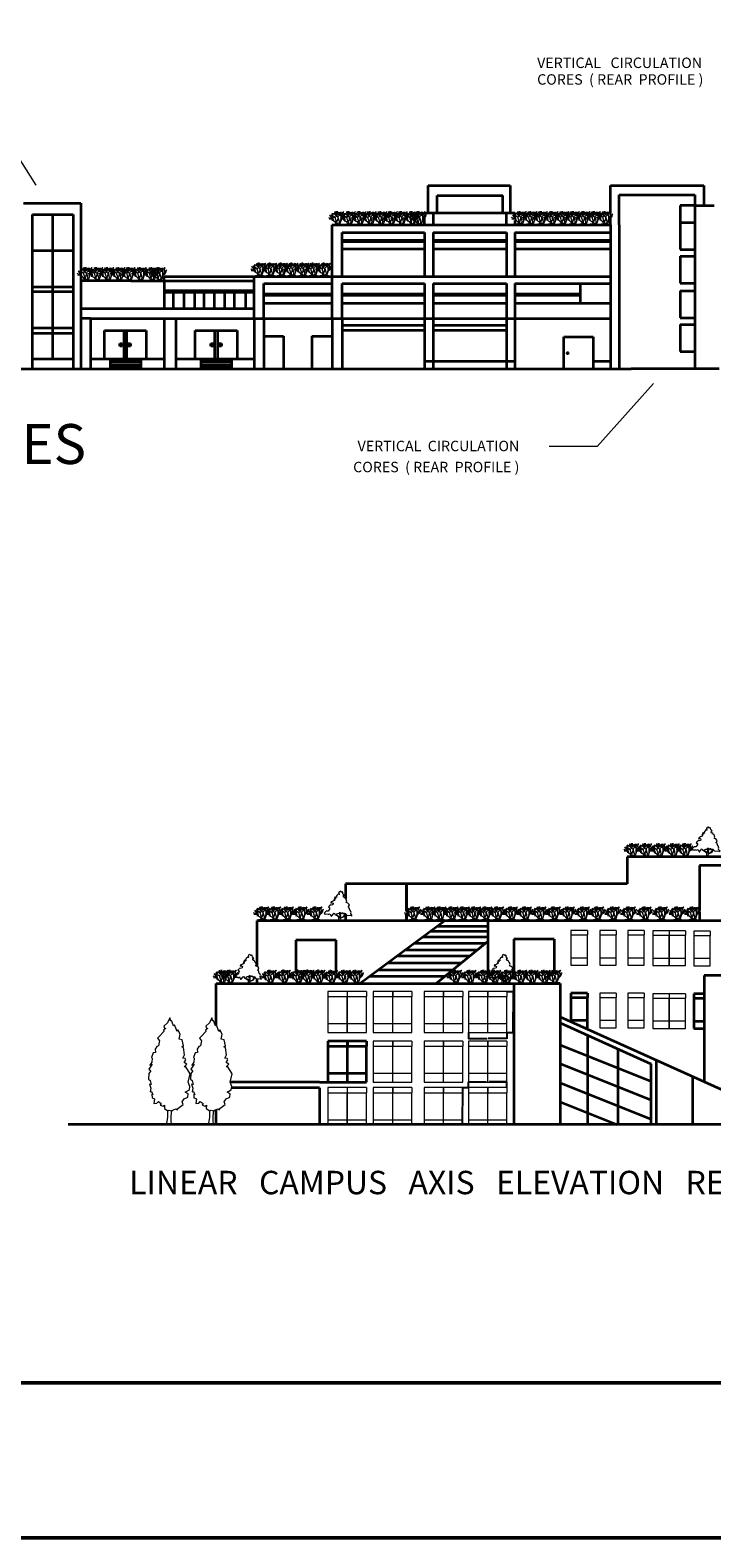
# Model space of a CAD drawing. Units: inches. Extents: x -1080 to 1950, y -1929 to 857.
# Tile 6 of 16: x 294 to 991, y -1929 to -389. Entities that reach past the tile are written whole.
import ezdxf

# ---------------------------------------------------------------- set-up
doc = ezdxf.new("R2010")
doc.units = ezdxf.units.IN
doc.header["$MEASUREMENT"] = 0
for name, color, linetype, lineweight in [('A-ANNO-DIMS', 2, 'Continuous', 18), ('A-ANNO-SYMB', 2, 'Continuous', 18), ('A-ANNO-TEXT', 7, 'Continuous', 25), ('A-ANNO-TTLB', 7, 'Continuous', 50), ('A-ELEV', 7, 'Continuous', 35), ('A-GLAZ', 4, 'Continuous', 18), ('L-PLNT', 82, 'Continuous', 13)]:
    doc.layers.add(name, color=color, linetype=linetype, lineweight=lineweight)
doc.styles.get("Standard").update_dxf_attribs({"font": 'arial.ttf'})
doc.dimstyles.get("Standard").update_dxf_attribs({"dimtxt": 0.18, "dimasz": 0.18, "dimexe": 0.18, "dimexo": 0.0625, "dimgap": 0.09, "dimtad": 0, "dimtih": 1, "dimtoh": 1, "dimdec": 4, "dimzin": 0, "dimdsep": 46, "dimtxsty": 'Standard', "dimcen": 0.09, "dimadec": 0, "dimazin": 0, "dimtfac": 1, "dimtdec": 4, "dimtofl": 0, "dimtmove": 0, "dimatfit": 3, "dimfxl": 1, "dimtolj": 1, "dimtzin": 0, "dimarcsym": 0})

# ---------------------------------------------------------------- blocks, each defined once
blk = doc.blocks.new('*U6')
for p, q in [((-451.104, 219.456), (-601.0402, 303.8094)), ((-451.104, 219.456), (-587.4512, 234.2388)), ((-463.296, 280.416), (-552.577, 423.037)), ((-463.296, 280.416), (-512.064, 292.608)), ((-329.184, 316.992), (-499.872, 414.528)), ((-353.568, 316.992), (-487.68, 377.952)), ((-426.72, 414.528), (-475.488, 475.488)), ((-402.336, 207.264), (-463.296, 280.416)), ((-414.528, 182.88), (-463.296, 182.88)), ((-377.952, 463.296), (-451.104, 487.68)), ((-426.72, 316.992), (-451.104, 329.184)), ((-377.952, 146.304), (-451.104, 219.456)), ((-402.336, 12.192), (-451.104, 0)), ((-426.72, 414.528), (-390.144, 499.872)), ((-426.72, 316.992), (-426.72, 414.528)), ((-402.336, 207.264), (-426.72, 316.992)), ((-377.952, 146.304), (-402.336, 207.264)), ((-341.376, 12.192), (-402.336, 12.192)), ((-377.952, 463.296), (-329.184, 524.256)), ((-207.264, 304.8), (-377.952, 463.296)), ((-329.184, 121.92), (-377.952, 146.304)), ((-329.184, 316.992), (-353.568, 316.992)), ((-243.84, 24.384), (-341.376, 12.192)), ((-338.455, 424.7896), (-290.3982, 464.5406)), ((-329.184, 316.992), (-207.264, 451.104)), ((-268.224, 109.728), (-329.184, 316.992)), ((-292.608, 60.96), (-329.184, 121.92)), ((-243.84, 24.384), (-329.184, 0)), ((-316.7634, 502.285), (-327.6092, 559.9176)), ((-296.5958, 484.4034), (-316.7634, 502.285)), ((-286.512, 498.3226), (-307.4416, 538.0736)), ((-305.8922, 396.9512), (-302.7934, 478.4344)), ((-304.3428, 426.7708), (-268.7066, 458.5716)), ((-302.7934, 478.4344), (-270.256, 518.1854)), ((-219.456, 24.384), (-292.608, 60.96)), ((-290.3982, 464.5406), (-265.6078, 577.8246)), ((-268.7066, 458.5716), (-250.0884, 500.3038)), ((-207.264, 451.104), (-268.224, 548.64)), ((-268.224, 109.728), (-219.456, 195.072)), ((-219.456, 48.768), (-268.224, 109.728)), ((-243.84, 24.384), (-195.072, 24.384)), ((-240.792, 502.285), (-228.3968, 573.8368)), ((-182.88, 499.872), (-219.456, 512.064)), ((-219.456, 195.072), (-207.264, 304.8)), ((-219.456, 24.384), (-109.728, 73.152)), ((-219.456, 24.384), (-158.496, 73.152)), ((-219.456, 24.384), (-219.456, 48.768)), ((-219.456, 24.384), (-73.152, 24.384)), ((-207.264, 451.104), (-134.112, 487.68)), ((-195.072, 316.992), (-182.88, 377.952)), ((-170.688, 219.456), (-195.072, 316.992)), ((-195.072, 24.384), (-158.496, 12.192)), ((-182.88, 499.872), (-158.496, 536.448)), ((-121.92, 414.528), (-182.88, 499.872)), ((-182.88, 377.952), (-97.536, 426.72)), ((-146.304, 134.112), (-170.688, 219.456)), ((-158.496, 73.152), (-146.304, 134.112)), ((-158.496, 12.192), (-85.344, 0)), ((-129.1844, 450.6214), (-140.0302, 542.036)), ((-134.112, 487.68), (-97.536, 548.64)), ((-85.7758, 389.001), (-129.1844, 452.6026)), ((-73.152, 329.184), (-109.728, 499.872)), ((-109.728, 73.152), (-48.768, 243.84)), ((-97.536, 426.72), (-24.384, 524.256)), ((-85.7758, 472.4908), (-73.3552, 548.005)), ((-70.2564, 426.7708), (-85.7758, 472.4908)), ((-85.344, 134.112), (-73.152, 329.184)), ((-73.152, 402.336), (-60.96, 512.064)), ((-24.384, 268.224), (-73.152, 402.336)), ((-73.152, 24.384), (0, 0)), ((-48.768, 243.84), (24.384, 304.8)), ((-12.9032, 555.9552), (-2.0574, 522.1732)), ((-12.192, 274.32), (8.7884, 335.3562)), ((-5.1562, 486.3846), (2.5908, 542.036)), ((8.7884, 335.3562), (-5.1562, 486.3846)), ((-3.6068, 492.3536), (14.986, 518.1854)), ((-0.508, 508.254), (22.7584, 536.067)), ((1.0414, 526.1356), (35.1536, 559.9176)), ((2.5908, 542.036), (21.209, 555.9552)), ((8.7884, 335.3562), (33.6042, 412.8516)), ((24.384, 304.8), (36.576, 390.144)), ((24.384, 304.8), (73.152, 377.952)), ((33.6042, 412.8516), (92.5068, 464.5406)), ((36.576, 390.144), (73.152, 438.912)), ((48.768, 341.376), (60.96, 390.144)), ((60.96, 390.144), (85.344, 414.528))]:
    blk.add_line(p, q)
blk = doc.blocks.new('*U2')
for points in [[(22.0124, 137.721), (18.5475, 141.5624), (15.5282, 138.2446), (13.8028, 139.3505), (13.3714, 142.1153), (11.2148, 143.2214), (8.1954, 140.4564), (4.7447, 141.0094), (2.1567, 136.0326), (2.1567, 131.6088), (5.6074, 129.9499), (3.0193, 128.2909), (0.4313, 130.5029), (-6.9015, 123.3141), (-6.9015, 121.6552), (-9.9208, 119.9963), (-9.0581, 118.3373), (-6.9015, 115.0195), (-10.7835, 112.2546), (-14.6656, 115.0195), (-16.8222, 114.4665), (-17.6849, 112.2546), (-14.6656, 111.7016), (-14.2342, 107.2778), (-17.6065, 107.8307), (-21.5669, 103.9599), (-17.2536, 103.4069), (-18.9789, 97.8771), (-22.8609, 97.3241), (-27.1743, 94.5593), (-32.3504, 91.7944), (-32.7817, 94.0063), (-36.6638, 85.7116), (-29.7624, 87.3705), (-25.449, 84.6056), (-26.743, 77.9699), (-34.507, 75.205), (-37.9578, 77.4169), (-39.2518, 74.099), (-42.2711, 73.5461), (-44.8592, 70.2282), (-47.8786, 66.3574), (-43.9965, 63.0395), (-41.4085, 64.6985), (-44.3346, 59.8898), (-42.2089, 60.1377), (-42.5159, 55.7849), (-49.6039, 46.4502), (-58.2307, 45.8972), (-62.1127, 43.6853), (-68.5828, 36.4966), (-65.9947, 32.0727), (-50.0352, 32.6257), (-47.0159, 30.4138), (-39.6831, 33.7317), (-34.507, 22.6721), (-32.3504, 22.6721), (-22.4296, 34.8376), (-19.4102, 36.4966), (-17.2536, 33.7317), (-17.2536, 29.8608), (-13.8028, 28.7549), (-9.0581, 28.7549), (-7.3328, 32.6257), (-1.7254, 35.3906), (3.8821, 35.9436), (6.4701, 38.1555), (6.9014, 38.7085), (8.1954, 41.4734), (9.9208, 40.3674), (11.2148, 35.9436), (14.2341, 37.6025), (15.0968, 36.4966), (15.9595, 33.7317), (18.9789, 38.7085), (21.9982, 38.7085), (23.2922, 36.4966), (21.9982, 34.2847), (25.4489, 35.3906), (26.743, 33.7317), (29.7623, 35.9436), (32.7817, 34.8376), (38.8204, 28.7549), (41.4084, 27.6489), (43.5651, 25.437), (61.6813, 27.0959), (65.132, 23.7781), (67.7201, 24.884), (60.8186, 33.7317), (60.3873, 37.0495), (62.544, 40.3674), (58.662, 50.874), (56.5053, 50.874), (52.1919, 66.3574), (47.8785, 66.9103), (50.4665, 69.1222), (53.9172, 77.9699), (47.0158, 85.1586), (38.3891, 87.9235), (42.2711, 94.0063)], [(42.2711, 94.0063), (38.8204, 104.5129), (36.6637, 104.5129), (32.3503, 113.9135), (29.7623, 113.3605), (26.743, 113.3605), (24.5862, 117.7844), (25.8802, 123.8671), (29.331, 123.8671), (22.8609, 131.6088), (21.9982, 137.6916)], [(-12.9401, 28.7549), (-2.588, 22.1191), (0.8626, 17.6953), (1.7253, 11.6125), (0, 0)], [(-9.9208, 28.2019), (0, 23.2251), (3.4507, 19.9072), (4.7447, 15.4834), (8.6267, 27.0959), (6.4701, 37.6025)], [(34.5071, 33.1787), (27.1743, 18.2483), (9.0581, 10.5066), (7.7641, 3.8708), (8.1954, 0)], [(8.1954, 40.3674), (11.2148, 27.6489), (8.1954, 13.8245), (24.5862, 19.9072), (32.7817, 34.2847)]]:
    blk.add_lwpolyline(points)
blk = doc.blocks.new('*U5')
blk.add_lwpolyline([(-2.754, 191.699), (-6.78, 182.851), (-13.682, 176.953), (-11.956, 173.266), (-9.656, 172.529), (-14.257, 170.317), (-13.682, 167.368), (-21.733, 157.783), (-25.184, 154.834), (-21.158, 150.41), (-21.733, 147.461), (-22.884, 140.825), (-26.334, 140.087), (-29.21, 134.926), (-28.635, 129.028), (-32.661, 128.291), (-36.111, 120.18), (-34.386, 118.706), (-35.536, 111.333), (-38.987, 106.171), (-34.386, 107.646), (-40.712, 98.798), (-37.261, 95.849), (-40.712, 90.688), (-41.287, 80.366), (-38.412, 78.154), (-36.686, 70.781), (-39.562, 71.518), (-37.261, 64.145), (-38.412, 57.509), (-36.111, 58.247), (-33.236, 52.348), (-35.536, 53.086), (-34.961, 46.45), (-30.36, 44.975), (-31.51, 36.128), (-26.334, 36.865), (-23.459, 39.814), (-18.283, 36.128), (-20.008, 33.178), (-14.832, 31.704), (-11.956, 33.178), (-12.531, 27.28), (-6.205, 22.856), (-3.905, 24.331), (0.121, 22.856), (8.173, 26.543), (11.624, 25.068), (12.199, 27.28), (21.4, 34.653), (19.675, 39.077), (23.701, 44.975), (30.027, 47.924), (30.602, 53.823), (25.426, 56.772), (32.903, 61.196), (34.053, 67.094), (30.602, 75.205), (34.628, 89.951), (26.576, 103.222), (23.701, 103.222), (28.302, 107.646), (23.701, 110.595), (26.576, 115.756), (25.426, 117.968), (20.825, 118.706), (24.276, 124.604), (22.551, 137.876), (19.1, 139.35), (22.551, 140.825), (19.675, 151.884), (14.499, 153.359), (16.224, 162.207), (12.199, 170.317), (10.473, 167.368), (5.872, 179.165), (4.147, 177.69), (0.696, 187.275), (-0.454, 185.8)], close=True)
for points in [[(-6.813, 23.669), (-6.813, 11.669), (-8.627, 0)], [(0.387, 23.669), (-0.576, 13.271), (-0.576, 3.686), (0, 0)]]:
    blk.add_lwpolyline(points)
blk = doc.blocks.new('WIN-TYPE-D')
for p, q in [((19.8, 41.9), (0, 41.9)), ((0, 41.9), (0, 36.7)), ((0, 36.7), (0, 9.1)), ((0, 36.7), (19.8, 36.7)), ((39.5, 41.9), (19.7, 41.9)), ((19.7, 41.9), (19.7, 36.7)), ((19.7, 36.7), (19.7, 9.1)), ((19.7, 36.7), (39.5, 36.7)), ((19.8, 41.9), (19.8, 36.7)), ((19.8, 9.1), (19.8, 36.7)), ((39.5, 41.9), (39.5, 36.7)), ((39.5, 9.1), (39.5, 36.7)), ((0, 9.1), (19.8, 9.1)), ((0, 9.1), (0, 0)), ((0, 0), (19.8, 0)), ((19.7, 9.1), (39.5, 9.1)), ((19.7, 9.1), (19.7, 0)), ((19.7, 0), (39.5, 0)), ((19.8, 0), (19.8, 9.1)), ((39.5, 0), (39.5, 9.1))]:
    blk.add_line(p, q)
blk = doc.blocks.new('WIN-TYPE-F')
for p, q in [((16.7, 35.4), (0, 35.4)), ((0, 35.4), (0, 31)), ((0, 31), (0, 7.7)), ((0, 31), (16.7, 31)), ((33.3, 35.4), (16.6, 35.4)), ((16.6, 35.4), (16.6, 31)), ((16.6, 31), (16.6, 7.7)), ((16.6, 31), (33.3, 31)), ((16.7, 35.4), (16.7, 31)), ((16.7, 7.7), (16.7, 31)), ((33.3, 35.4), (33.3, 31)), ((33.3, 7.7), (33.3, 31)), ((0, 7.7), (16.7, 7.7)), ((0, 7.7), (0, 0)), ((0, 0), (16.7, 0)), ((16.6, 7.7), (33.3, 7.7)), ((16.6, 7.7), (16.6, 0)), ((16.6, 0), (33.3, 0)), ((16.7, 0), (16.7, 7.7)), ((33.3, 0), (33.3, 7.7))]:
    blk.add_line(p, q)
blk = doc.blocks.new('WIN-TYPE-J')
for p, q in [((19.8, 37.7), (0, 37.7)), ((0, 37.7), (0, 32.5)), ((0, 32.5), (0, 4.9)), ((0, 32.5), (19.8, 32.5)), ((39.5, 37.7), (19.7, 37.7)), ((19.7, 37.7), (19.7, 32.5)), ((19.7, 32.5), (19.7, 4.9)), ((19.7, 32.5), (39.5, 32.5)), ((19.8, 37.7), (19.8, 32.5)), ((19.8, 4.9), (19.8, 32.5)), ((39.5, 37.7), (39.5, 32.5)), ((39.5, 4.9), (39.5, 32.5)), ((0, 4.9), (19.8, 4.9)), ((0, 4.9), (0, 0)), ((19.7, 4.9), (39.5, 4.9)), ((19.7, 4.9), (19.7, 0)), ((19.8, 0), (19.8, 4.9)), ((39.5, 0), (39.5, 4.9))]:
    blk.add_line(p, q)
blk = doc.blocks.new('WIN-TYPE-K')
for p, q in [((16.7, 35.4), (0, 35.4)), ((0, 35.4), (0, 31)), ((0, 31), (0, 7.7)), ((0, 31), (16.7, 31)), ((16.7, 35.4), (16.7, 31)), ((16.7, 7.7), (16.7, 31)), ((0, 7.7), (16.7, 7.7)), ((0, 7.7), (0, 0)), ((0, 0), (16.7, 0)), ((16.7, 0), (16.7, 7.7))]:
    blk.add_line(p, q)
blk = doc.blocks.new('*D41')
at = {"layer": 'A-ANNO-DIMS', "color": 0, "lineweight": -2, "transparency": 16777216}
for p, q in [((781.3, -1370.7), (787.7, -1370.7)), ((787.5, -1370.8), (787.5, -1391.5)), ((787.5, -1412.4), (787.5, -1391.8)), ((781.3, -1412.6), (787.7, -1412.6))]:
    blk.add_line(p, q, dxfattribs=at)
at = {"layer": 'A-ANNO-DIMS', "color": 0, "transparency": 16777216}
for points in [[(787.5, -1370.8), (787.5, -1370.8), (787.5, -1370.7)], [(787.5, -1412.4), (787.5, -1412.4), (787.5, -1412.6)]]:
    blk.add_solid(points, dxfattribs=at)
at = {"layer": 'Defpoints', "color": 0, "transparency": 16777216}
for p in [(781.2, -1370.7), (787.5, -1370.7), (781.2, -1412.6)]:
    blk.add_point(p, dxfattribs=at)
at = {"layer": 'A-ANNO-DIMS', "color": 0, "transparency": 16777216, "insert": (787.5, -1391.6), "char_height": 0.18, "attachment_point": 5}
blk.add_mtext('\\A1;WINDOW TYPE D 42 TYP.', dxfattribs=at)
blk = doc.blocks.new('*D42')
at = {"layer": 'A-ANNO-DIMS', "color": 0, "lineweight": -2, "transparency": 16777216}
for p, q in [((741.7, -1412.7), (741.7, -1419.1)), ((781.2, -1412.7), (781.2, -1419.1)), ((741.9, -1418.9), (760.9, -1418.9)), ((781, -1418.9), (762, -1418.9))]:
    blk.add_line(p, q, dxfattribs=at)
at = {"layer": 'A-ANNO-DIMS', "color": 0, "transparency": 16777216}
for points in [[(741.9, -1418.9), (741.9, -1418.9), (741.7, -1418.9)], [(781, -1418.9), (781, -1418.9), (781.2, -1418.9)]]:
    blk.add_solid(points, dxfattribs=at)
at = {"layer": 'Defpoints', "color": 0, "transparency": 16777216}
for p in [(741.7, -1412.6), (781.2, -1412.6), (781.2, -1418.9)]:
    blk.add_point(p, dxfattribs=at)
at = {"layer": 'A-ANNO-DIMS', "color": 0, "transparency": 16777216, "insert": (761.5, -1418.9), "char_height": 0.18, "attachment_point": 5}
blk.add_mtext('\\A1;39 TYP.', dxfattribs=at)
blk = doc.blocks.new('*D51')
at = {"layer": 'A-ANNO-DIMS', "color": 0, "lineweight": -2, "transparency": 16777216}
for p, q in [((741.7, -1469), (741.7, -1462.9)), ((741.9, -1463.1), (759.9, -1463.1)), ((781, -1463.1), (763, -1463.1)), ((781.2, -1469), (781.2, -1462.9))]:
    blk.add_line(p, q, dxfattribs=at)
at = {"layer": 'A-ANNO-DIMS', "color": 0, "transparency": 16777216}
for points in [[(741.9, -1463.1), (741.9, -1463.2), (741.7, -1463.1)], [(781, -1463.1), (781, -1463.2), (781.2, -1463.1)]]:
    blk.add_solid(points, dxfattribs=at)
at = {"layer": 'Defpoints', "color": 0, "transparency": 16777216}
for p in [(781.2, -1463.1), (741.7, -1469.1), (781.2, -1469.1)]:
    blk.add_point(p, dxfattribs=at)
at = {"layer": 'A-ANNO-DIMS', "color": 0, "transparency": 16777216, "insert": (761.5, -1463.1), "char_height": 0.18, "attachment_point": 5}
blk.add_mtext('\\A1;WINDOW TYPE J 39 TYP.', dxfattribs=at)
blk = doc.blocks.new('*D52')
at = {"layer": 'A-ANNO-DIMS', "color": 0, "lineweight": -2, "transparency": 16777216}
for p, q in [((741.7, -1469.1), (735.6, -1469.1)), ((735.8, -1469.2), (735.8, -1487.7)), ((735.8, -1506.5), (735.8, -1488.1)), ((741.7, -1506.7), (735.6, -1506.7))]:
    blk.add_line(p, q, dxfattribs=at)
at = {"layer": 'A-ANNO-DIMS', "color": 0, "transparency": 16777216}
for points in [[(735.8, -1469.2), (735.8, -1469.2), (735.8, -1469.1)], [(735.8, -1506.5), (735.8, -1506.5), (735.8, -1506.7)]]:
    blk.add_solid(points, dxfattribs=at)
at = {"layer": 'Defpoints', "color": 0, "transparency": 16777216}
for p in [(735.8, -1469.1), (741.7, -1469.1), (741.7, -1506.7)]:
    blk.add_point(p, dxfattribs=at)
at = {"layer": 'A-ANNO-DIMS', "color": 0, "transparency": 16777216, "insert": (735.8, -1487.9), "char_height": 0.18, "attachment_point": 5}
blk.add_mtext('\\A1;38 TYP.', dxfattribs=at)

msp = doc.modelspace()

# ---------------------------------------------------------------- linework, layer by layer
at = {"layer": 'A-ANNO-SYMB'}
for p, q in [((299.9, -547), (254.9, -475.5)), ((930.9, -749.5), (873.4, -814)), ((873.4, -814), (824.4, -814))]:
    msp.add_line(p, q, dxfattribs=at)
at = {"layer": 'A-ANNO-TTLB'}
for points in [[(-1080.1, 856.5), (1950.4, 856.5), (1950.4, -1929), (-1080.1, -1929)], [(-957.6, 743.5), (1813.4, 743.5), (1813.4, -1770.5), (-957.6, -1770.5)]]:
    msp.add_lwpolyline(points, close=True, dxfattribs=at)
at = {"layer": 'A-ELEV'}
for p, q in [((700.8, -575.1), (700.8, -547.3)), ((700.8, -547.3), (784.5, -547.3)), ((784.5, -547.3), (784.5, -575.1)), ((887.1, -574.6), (887.1, -547.3)), ((887.1, -547.3), (982.2, -547.3)), ((982.2, -547.3), (982.2, -567.8)), ((287.1, -565.3), (345.7, -565.3)), ((345.7, -565.3), (345.7, -632.8)), ((709.8, -575.1), (709.8, -557.6)), ((709.8, -557.6), (776.9, -557.6)), ((776.9, -575.1), (776.9, -557.6)), ((895.7, -587.4), (895.7, -556.7)), ((895.7, -556.7), (973, -556.7)), ((973, -567.8), (958.2, -567.8)), ((958.2, -567.8), (958.2, -585.2)), ((973, -556.7), (973, -734.7)), ((973, -567.8), (992.9, -567.8)), ((296.3, -734.7), (296.3, -576.7)), ((296.3, -576.7), (338, -576.7)), ((316.6, -576.7), (316.6, -724.3)), ((338, -576.7), (338, -734.7)), ((697, -575.1), (700.8, -575.1)), ((697, -575.1), (697, -575.1)), ((697, -579.3), (697, -579.2)), ((697, -587.4), (697, -580.4)), ((700.8, -575.1), (775.9, -575.1)), ((705.6, -575.1), (705.6, -587.4)), ((775.9, -575.1), (789.3, -575.1)), ((780.7, -587.4), (780.7, -575.1)), ((789.3, -575.1), (789.3, -576.3)), ((789.3, -581.9), (789.3, -582)), ((789.3, -582.9), (789.3, -587.4)), ((887.1, -576), (887.1, -575.1)), ((887.1, -587.4), (887.1, -580.1)), ((958.2, -585.2), (973, -585.2)), ((958.2, -585.2), (958.2, -612.7)), ((602.5, -683), (602.5, -587.4)), ((602.5, -587.4), (697, -587.4)), ((612.7, -595.4), (697, -595.4)), ((612.7, -640.1), (612.7, -595.4)), ((697, -587.4), (887.1, -587.4)), ((697, -595.4), (697, -640.1)), ((705.6, -595.4), (705.6, -640.1)), ((705.6, -595.4), (780.7, -595.4)), ((780.7, -595.4), (780.7, -640.1)), ((789.3, -595.4), (789.3, -640.1)), ((789.3, -595.4), (887.1, -595.4)), ((887.1, -587.4), (887.1, -734.7)), ((895.7, -587.4), (895.7, -734.7)), ((296.3, -613.5), (338, -613.5)), ((612.7, -603.1), (697, -603.1)), ((612.7, -604.6), (697, -604.6)), ((612.7, -612), (697, -612)), ((705.6, -603.1), (780.7, -603.1)), ((705.6, -604.6), (780.7, -604.6)), ((705.6, -612), (780.7, -612)), ((789.3, -603.1), (887.1, -603.1)), ((789.3, -604.6), (887.1, -604.6)), ((789.3, -612), (887.1, -612)), ((958.2, -612.7), (973, -612.7)), ((958.2, -619.4), (973, -619.4)), ((958.2, -619.4), (958.2, -646.9)), ((345.7, -639.3), (345.7, -734.7)), ((396.7, -644.6), (345.7, -644.6)), ((396.7, -644.6), (421.4, -644.6)), ((421.4, -644.6), (430.8, -644.6)), ((430.8, -644.6), (430.8, -640.1)), ((430.8, -640.1), (522.7, -640.1)), ((430.8, -644.6), (430.8, -672.9)), ((430.8, -644.6), (522.7, -644.6)), ((522.7, -683), (522.7, -640.1)), ((522.7, -640.1), (602.5, -640.1)), ((602.5, -647.5), (602.5, -640.1)), ((602.5, -640.1), (887.1, -640.1)), ((868.3, -640.1), (887.1, -640.1)), ((958.2, -646.9), (973, -646.9)), ((296.3, -650.7), (338, -650.7)), ((296.3, -655.4), (338, -655.4)), ((430.8, -654.4), (522.7, -654.4)), ((437.5, -656.5), (430.8, -656.5)), ((522.7, -656.5), (437.5, -656.5)), ((437.5, -656.5), (437.5, -656.5)), ((440.3, -672.9), (440.3, -656.5)), ((451.2, -672.9), (451.2, -656.5)), ((462.1, -672.9), (462.1, -656.5)), ((471.8, -672.9), (471.8, -656.5)), ((482.4, -672.9), (482.4, -656.5)), ((492.9, -672.9), (492.9, -656.5)), ((502.7, -672.9), (502.7, -656.5)), ((514.2, -672.9), (514.2, -656.5)), ((522.7, -672.9), (522.7, -656.5)), ((522.7, -672.9), (522.7, -656.5)), ((532.7, -683), (532.7, -647.5)), ((532.7, -647.5), (602.5, -647.5)), ((532.7, -657.9), (602.5, -657.9)), ((532.7, -659.4), (602.5, -659.4)), ((612.7, -683), (612.7, -647.5)), ((612.7, -647.5), (697, -647.5)), ((612.7, -657.9), (697, -657.9)), ((612.7, -659.4), (697, -659.4)), ((697, -647.5), (697, -734.7)), ((705.6, -647.5), (780.7, -647.5)), ((705.6, -647.5), (705.6, -734.7)), ((705.6, -657.9), (780.7, -657.9)), ((705.6, -659.4), (780.7, -659.4)), ((780.7, -647.5), (780.7, -734.7)), ((789.3, -647.5), (887.1, -647.5)), ((789.3, -647.5), (789.3, -734.7)), ((789.3, -657.9), (856.2, -657.9)), ((789.3, -659.4), (856.2, -659.4)), ((856.2, -667.6), (856.2, -647.5)), ((958.2, -654.8), (973, -654.8)), ((958.2, -654.8), (958.2, -682.3)), ((345.7, -672.9), (522.7, -672.9)), ((532.7, -667.6), (602.5, -667.6)), ((612.7, -667.6), (697, -667.6)), ((705.6, -667.6), (780.7, -667.6)), ((789.3, -667.6), (887.1, -667.6)), ((296.3, -692.6), (338, -692.6)), ((355.6, -683), (345.7, -683)), ((355.6, -683), (532.4, -683)), ((355.6, -683), (355.6, -734.7)), ((430.8, -683), (430.8, -734.7)), ((442.8, -683), (442.8, -734.7)), ((522.7, -683), (522.7, -734.7)), ((532.7, -683), (532.7, -734.7)), ((532.7, -683), (887.1, -683)), ((602.5, -683), (602.5, -734.7)), ((612.7, -683), (612.7, -734.7)), ((612.7, -689.9), (697, -689.9)), ((705.6, -689.9), (780.7, -689.9)), ((958.2, -682.3), (973, -682.3)), ((958.2, -689.2), (973, -689.2)), ((958.2, -689.2), (958.2, -716.7)), ((296.3, -698.1), (338, -698.1)), ((369.8, -724.3), (369.8, -695.5)), ((369.8, -695.5), (411.4, -695.5)), ((389.9, -724.3), (389.9, -695.5)), ((392.8, -724.3), (392.8, -695.5)), ((411.4, -695.5), (412.6, -695.5)), ((412.6, -695.5), (412.6, -724.3)), ((462.5, -724.3), (462.5, -695.5)), ((462.5, -695.5), (504.2, -695.5)), ((482.7, -724.3), (482.7, -695.5)), ((485.6, -724.3), (485.6, -695.5)), ((504.2, -695.5), (505.4, -695.5)), ((505.4, -695.5), (505.4, -724.3)), ((532.7, -701.3), (552.9, -701.3)), ((552.9, -701.3), (552.9, -734.7)), ((581.6, -701.3), (602.5, -701.3)), ((581.6, -701.3), (581.6, -734.7)), ((612.7, -695), (697, -695)), ((705.6, -695), (780.7, -695)), ((839.4, -734.7), (839.4, -701.9)), ((839.4, -701.9), (869.1, -701.9)), ((869.1, -701.9), (869.1, -734.7)), ((385.6, -708.8), (388.1, -708.8)), ((385.6, -711.4), (385.6, -708.8)), ((388.1, -711.4), (385.6, -711.4)), ((388.1, -708.8), (388.1, -711.4)), ((394.2, -708.8), (396.6, -708.8)), ((394.2, -711.4), (394.2, -708.8)), ((396.6, -711.4), (394.2, -711.4)), ((396.6, -708.8), (396.6, -711.4)), ((478.4, -708.8), (480.9, -708.8)), ((478.4, -711.4), (478.4, -708.8)), ((480.9, -711.4), (478.4, -711.4)), ((480.9, -708.8), (480.9, -711.4)), ((487, -708.8), (489.4, -708.8)), ((487, -711.4), (487, -708.8)), ((489.4, -711.4), (487, -711.4)), ((489.4, -708.8), (489.4, -711.4)), ((958.2, -716.7), (973, -716.7)), ((-262.7, -734.7), (342.8, -734.7)), ((296.3, -724.3), (338, -724.3)), ((342.8, -734.7), (908.2, -734.7)), ((355.6, -724.3), (430.8, -724.3)), ((375.9, -734.7), (375.9, -724.3)), ((375.9, -727), (407.3, -727)), ((375.9, -730), (407.3, -730)), ((375.9, -732.2), (407.3, -732.2)), ((407.3, -734.7), (407.3, -724.3)), ((442.8, -724.3), (507, -724.3)), ((468.7, -734.7), (468.7, -724.3)), ((468.7, -727), (500, -727)), ((468.7, -727), (500, -727)), ((468.7, -730), (500, -730)), ((468.7, -732.2), (500, -732.2)), ((500, -734.7), (500, -724.3)), ((507, -724.3), (522.7, -724.3)), ((697, -726.7), (789.3, -726.7)), ((869.1, -726.7), (887.1, -726.7)), ((998.1, -734.7), (908.2, -734.7)), ((982.2, -734.7), (971, -734.7)), ((903.9, -1233.3), (903.9, -1260.7)), ((1191.2, -1233.3), (903.9, -1233.3)), ((1182.7, -1242), (977.9, -1242)), ((977.9, -1242), (977.9, -1287.4)), ((616.2, -1260.7), (616.2, -1275.9)), ((678.4, -1260.7), (616.2, -1260.7)), ((903.9, -1260.7), (676.1, -1260.7)), ((678.4, -1260.7), (678.4, -1288.5)), ((678.4, -1288.5), (678.4, -1260.7)), ((616.2, -1291.7), (616.2, -1298.5)), ((616.2, -1293.9), (616.2, -1296.9)), ((678.4, -1292.3), (678.4, -1298.5)), ((678.4, -1298.5), (678.4, -1292.3)), ((977.9, -1289.3), (977.9, -1298.5)), ((977.9, -1298.5), (525.5, -1298.5)), ((525.5, -1298.5), (525.5, -1344.9)), ((717.7, -1298.5), (631.2, -1362.7)), ((703.3, -1309.2), (761.8, -1309.2)), ((710.1, -1304.1), (761.8, -1304.1)), ((761.8, -1354.1), (761.8, -1298.5)), ((1118.6, -1298.5), (977.9, -1298.5)), ((606.7, -1318.2), (565.5, -1318.2)), ((565.5, -1318.2), (565.5, -1349.3)), ((606.7, -1350.2), (606.7, -1318.2)), ((686.8, -1321.4), (759.3, -1321.4)), ((695.4, -1315), (761.8, -1315)), ((761.8, -1319.4), (708.8, -1362.7)), ((829.3, -1317.2), (788.1, -1317.2)), ((788.1, -1317.2), (788.1, -1352.3)), ((829.3, -1317.2), (829.3, -1352.6)), ((669.3, -1334.4), (743.4, -1334.4)), ((677.8, -1328.1), (751.2, -1328.1)), ((565.5, -1351.8), (565.5, -1352.4)), ((565.5, -1354.6), (565.5, -1355.1)), ((641.3, -1355.2), (717.9, -1355.2)), ((650, -1348.7), (725.9, -1348.7)), ((659.6, -1341.6), (734.6, -1341.6)), ((1118.6, -1354.5), (982.8, -1354.5)), ((982.8, -1354.5), (982.8, -1358.1)), ((484, -1405.1), (484, -1362.7)), ((484, -1362.7), (834.8, -1362.7)), ((525.5, -1357.6), (525.5, -1362.7)), ((606.7, -1356.9), (606.7, -1355.6)), ((606.7, -1362.7), (606.7, -1362.5)), ((761.8, -1362.7), (761.8, -1362)), ((788.1, -1362.7), (788.1, -1506.7)), ((835.6, -1362.7), (821.6, -1362.7)), ((829.3, -1361.7), (829.3, -1362)), ((835.6, -1362.7), (834.8, -1362.7)), ((835.6, -1362.7), (835.6, -1506.7)), ((982.8, -1358.1), (982.8, -1463.1)), ((863.3, -1372.5), (846.6, -1372.5)), ((846.6, -1372.5), (846.6, -1376.9)), ((846.6, -1376.9), (846.6, -1400.1)), ((846.6, -1376.9), (863.3, -1376.9)), ((863.3, -1372.5), (863.3, -1376.9)), ((863.3, -1400.1), (863.3, -1376.9)), ((982.8, -1373.2), (972.2, -1373.2)), ((972.2, -1373.2), (972.2, -1377.6)), ((972.2, -1377.6), (972.2, -1400.9)), ((972.2, -1377.6), (982.8, -1377.6)), ((835.6, -1396.7), (1079.5, -1506.7)), ((846.6, -1400.1), (863.3, -1400.1)), ((846.6, -1400.1), (846.6, -1401.7)), ((863.3, -1407.9), (863.3, -1400.1)), ((972.2, -1400.9), (982.8, -1400.9)), ((972.2, -1400.9), (972.2, -1408.6)), ((431.2, -1407.8), (431.2, -1408)), ((431.3, -1408), (431.2, -1408)), ((835.6, -1402.7), (928.2, -1444.7)), ((860.3, -1407.9), (863.3, -1407.9)), ((863.3, -1415.3), (863.3, -1506.7)), ((972.2, -1408.6), (982.8, -1408.6)), ((618.1, -1421.5), (598.2, -1421.5)), ((598.2, -1421.5), (598.2, -1426.7)), ((598.2, -1426.7), (598.2, -1454.3)), ((598.2, -1426.7), (618.1, -1426.7)), ((637.7, -1421.5), (617.9, -1421.5)), ((617.9, -1421.5), (617.9, -1426.7)), ((617.9, -1426.7), (617.9, -1454.3)), ((617.9, -1426.7), (637.7, -1426.7)), ((618.1, -1421.5), (618.1, -1426.7)), ((618.1, -1454.3), (618.1, -1426.7)), ((637.7, -1421.5), (637.7, -1426.7)), ((637.7, -1454.3), (637.7, -1426.7)), ((835.6, -1425.1), (928.2, -1462.3)), ((894.4, -1429.4), (894.4, -1506.7)), ((835.5, -1444.2), (928.2, -1481.5)), ((928.2, -1438.3), (928.2, -1438.5)), ((928.2, -1444.7), (928.2, -1506.7)), ((933.5, -1440.9), (933.5, -1506.7)), ((589.7, -1463.4), (498.3, -1463.4)), ((589.7, -1463.4), (598.2, -1463.4)), ((598.2, -1454.3), (618.1, -1454.3)), ((598.2, -1454.3), (598.2, -1463.4)), ((598.2, -1463.4), (618.1, -1463.4)), ((617.9, -1454.3), (637.7, -1454.3)), ((617.9, -1454.3), (617.9, -1463.4)), ((617.9, -1463.4), (637.7, -1463.4)), ((618.1, -1463.4), (618.1, -1454.3)), ((637.7, -1463.4), (637.7, -1454.3)), ((970.9, -1457.7), (970.9, -1506.7)), ((589.7, -1469.1), (499.9, -1469.1)), ((589.7, -1469.1), (589.7, -1506.7)), ((835, -1463.7), (927.7, -1501)), ((484, -1506.7), (484, -1491.4)), ((835.6, -1483.4), (893.5, -1506.7)), ((1612.5, -1506.7), (332.8, -1506.7))]:
    msp.add_line(p, q, dxfattribs=at)
msp.add_circle((843.2, -718.5), 0.635, dxfattribs=at)

# ---------------------------------------------------------------- block references
at = {"layer": 'A-GLAZ'}
for name, p in [('WIN-TYPE-K', (846.6, -1343.9)), ('WIN-TYPE-K', (876, -1343.9)), ('WIN-TYPE-K', (904.7, -1343.9)), ('WIN-TYPE-F', (930.3, -1344.3)), ('WIN-TYPE-K', (972.2, -1344.5)), ('WIN-TYPE-D', (598.2, -1412.6)), ('WIN-TYPE-D', (644.6, -1412.6)), ('WIN-TYPE-D', (696.4, -1412.6)), ('WIN-TYPE-D', (741.7, -1412.6)), ('WIN-TYPE-K', (876, -1407.9)), ('WIN-TYPE-K', (904.7, -1407.9)), ('WIN-TYPE-F', (930.3, -1408.4)), ('WIN-TYPE-D', (644.6, -1463.4)), ('WIN-TYPE-D', (696.4, -1463.4)), ('WIN-TYPE-D', (741.7, -1463.4)), ('WIN-TYPE-J', (598.2, -1506.7)), ('WIN-TYPE-J', (644.6, -1506.7)), ('WIN-TYPE-J', (696.4, -1506.7)), ('WIN-TYPE-J', (741.7, -1506.7))]:
    msp.add_blockref(name, p, dxfattribs=at)
at = {"layer": 'L-PLNT'}
for name, p, xscale, yscale, zscale in [('*U6', (613.5, -587.4), 0.0240303115076123, 0.0240303115076123, 0.0240303115076123), ('*U6', (625.4, -587.4), 0.0240303115076123, 0.0240303115076123, 0.0240303115076123), ('*U6', (636.3, -587.4), 0.0240303115076123, 0.0240303115076123, 0.0240303115076123), ('*U6', (647, -587.4), 0.0240303115076123, 0.0240303115076123, 0.0240303115076123), ('*U6', (657.9, -587.4), 0.0240303115076123, 0.0240303115076123, 0.0240303115076123), ('*U6', (668.3, -587.4), 0.0240303115076123, 0.0240303115076123, 0.0240303115076123), ('*U6', (678.8, -587.4), 0.0240303115076123, 0.0240303115076123, 0.0240303115076123), ('*U6', (689.7, -587.4), 0.0240303115076123, 0.0240303115076123, 0.0240303115076123), ('*U6', (696.8, -587.4), 0.0240303115076123, 0.0240303115076123, 0.0240303115076123), ('*U6', (800.3, -587.2), 0.0240303115076123, 0.0240303115076123, 0.0240303115076123), ('*U6', (811.2, -587.2), 0.0240303115076123, 0.0240303115076123, 0.0240303115076123), ('*U6', (821.9, -587.2), 0.0240303115076123, 0.0240303115076123, 0.0240303115076123), ('*U6', (832.8, -587.2), 0.0240303115076123, 0.0240303115076123, 0.0240303115076123), ('*U6', (843.8, -587.2), 0.0240303115076123, 0.0240303115076123, 0.0240303115076123), ('*U6', (854.5, -587.2), 0.0240303115076123, 0.0240303115076123, 0.0240303115076123), ('*U6', (865.4, -587.2), 0.0240303115076123, 0.0240303115076123, 0.0240303115076123), ('*U6', (876, -587.2), 0.0240303115076123, 0.0240303115076123, 0.0240303115076123), ('*U6', (887.1, -587.2), 0.0240303115076123, 0.0240303115076123, 0.0240303115076123), ('*U6', (356.5, -644.5), 0.0240303115076123, 0.0240303115076123, 0.0240303115076123), ('*U6', (367.5, -644.5), 0.0240303115076123, 0.0240303115076123, 0.0240303115076123), ('*U6', (378.6, -644.5), 0.0240303115076123, 0.0240303115076123, 0.0240303115076123), ('*U6', (390.2, -644.5), 0.0240303115076123, 0.0240303115076123, 0.0240303115076123), ('*U6', (400.5, -644.5), 0.0240303115076123, 0.0240303115076123, 0.0240303115076123), ('*U6', (411.9, -644.5), 0.0240303115076123, 0.0240303115076123, 0.0240303115076123), ('*U6', (423.8, -644.5), 0.0240303115076123, 0.0240303115076123, 0.0240303115076123), ('*U6', (431.2, -644.5), 0.0240303115076123, 0.0240303115076123, 0.0240303115076123), ('*U6', (533.8, -639.9), 0.0240303115076123, 0.0240303115076123, 0.0240303115076123), ('*U6', (545, -639.9), 0.0240303115076123, 0.0240303115076123, 0.0240303115076123), ('*U6', (556.2, -639.9), 0.0240303115076123, 0.0240303115076123, 0.0240303115076123), ('*U6', (567, -639.9), 0.0240303115076123, 0.0240303115076123, 0.0240303115076123), ('*U6', (578.1, -639.9), 0.0240303115076123, 0.0240303115076123, 0.0240303115076123), ('*U6', (588.7, -639.9), 0.0240303115076123, 0.0240303115076123, 0.0240303115076123), ('*U6', (600.1, -639.9), 0.0240303115076123, 0.0240303115076123, 0.0240303115076123), ('*U2', (984.7, -1232.7), 0.2096355800251992, 0.2096355800251992, 0.2096355800251992), ('*U6', (915.1, -1233.2), 0.024256363829807, 0.024256363829807, 0.024256363829807), ('*U6', (928.4, -1233.2), 0.024256363829807, 0.024256363829807, 0.024256363829807), ('*U6', (942.4, -1233.2), 0.024256363829807, 0.024256363829807, 0.024256363829807), ('*U6', (956.7, -1233.2), 0.024256363829807, 0.024256363829807, 0.024256363829807), ('*U6', (969, -1233.2), 0.024256363829807, 0.024256363829807, 0.024256363829807), ('*U2', (608.8, -1298.4), 0.2096355800251992, 0.2096355800251992, 0.2096355800251992), ('*U6', (536.9, -1297.8), 0.024256363829807, 0.024256363829807, 0.024256363829807), ('*U6', (549.1, -1297.8), 0.024256363829807, 0.024256363829807, 0.024256363829807), ('*U6', (562.2, -1297.8), 0.024256363829807, 0.024256363829807, 0.024256363829807), ('*U6', (576.3, -1297.8), 0.024256363829807, 0.024256363829807, 0.024256363829807), ('*U6', (591.4, -1297.8), 0.024256363829807, 0.024256363829807, 0.024256363829807), ('*U6', (691.2, -1297.8), 0.024256363829807, 0.024256363829807, 0.024256363829807), ('*U6', (707, -1297.8), 0.024256363829807, 0.024256363829807, 0.024256363829807), ('*U6', (718.3, -1297.8), 0.024256363829807, 0.024256363829807, 0.024256363829807), ('*U6', (730.4, -1297.8), 0.024256363829807, 0.024256363829807, 0.024256363829807), ('*U6', (741.9, -1297.8), 0.024256363829807, 0.024256363829807, 0.024256363829807), ('*U6', (753.5, -1297.8), 0.024256363829807, 0.024256363829807, 0.024256363829807), ('*U6', (765.1, -1297.8), 0.024256363829807, 0.024256363829807, 0.024256363829807), ('*U6', (777, -1297.8), 0.024256363829807, 0.024256363829807, 0.024256363829807), ('*U6', (791.2, -1297.8), 0.024256363829807, 0.024256363829807, 0.024256363829807), ('*U6', (805.5, -1297.8), 0.024256363829807, 0.024256363829807, 0.024256363829807), ('*U6', (820.4, -1297.8), 0.024256363829807, 0.024256363829807, 0.024256363829807), ('*U6', (834.9, -1297.8), 0.024256363829807, 0.024256363829807, 0.024256363829807), ('*U6', (849.4, -1297.8), 0.024256363829807, 0.024256363829807, 0.024256363829807), ('*U6', (864.7, -1297.8), 0.024256363829807, 0.024256363829807, 0.024256363829807), ('*U6', (879.2, -1297.8), 0.024256363829807, 0.024256363829807, 0.024256363829807), ('*U6', (895.3, -1297.8), 0.024256363829807, 0.024256363829807, 0.024256363829807), ('*U6', (911.5, -1297.8), 0.024256363829807, 0.024256363829807, 0.024256363829807), ('*U6', (927.8, -1297.8), 0.024256363829807, 0.024256363829807, 0.024256363829807), ('*U6', (944.3, -1297.8), 0.024256363829807, 0.024256363829807, 0.024256363829807), ('*U6', (961, -1297.8), 0.024256363829807, 0.024256363829807, 0.024256363829807), ('*U6', (976.7, -1297.8), 0.024256363829807, 0.024256363829807, 0.024256363829807), ('*U2', (516.2, -1363), 0.2096355800251992, 0.2096355800251992, 0.2096355800251992), ('*U2', (775.7, -1363), 0.2096355800251992, 0.2096355800251992, 0.2096355800251992), ('*U6', (495.5, -1362.6), 0.024256363829807, 0.024256363829807, 0.024256363829807), ('*U6', (503.8, -1362.6), 0.024256363829807, 0.024256363829807, 0.024256363829807), ('*U6', (544.7, -1362.6), 0.024256363829807, 0.024256363829807, 0.024256363829807), ('*U6', (559, -1362.4), 0.024256363829807, 0.024256363829807, 0.024256363829807), ('*U6', (573.4, -1362.4), 0.024256363829807, 0.024256363829807, 0.024256363829807), ('*U6', (583.4, -1362.4), 0.024256363829807, 0.024256363829807, 0.024256363829807), ('*U6', (594.6, -1362.4), 0.024256363829807, 0.024256363829807, 0.024256363829807), ('*U6', (607.4, -1362.8), 0.024256363829807, 0.024256363829807, 0.024256363829807), ('*U6', (620.5, -1362.5), 0.024256363829807, 0.024256363829807, 0.024256363829807), ('*U6', (632.4, -1362.5), 0.024256363829807, 0.024256363829807, 0.024256363829807), ('*U6', (734.1, -1362.5), 0.024256363829807, 0.024256363829807, 0.024256363829807), ('*U6', (748.9, -1362.5), 0.024256363829807, 0.024256363829807, 0.024256363829807), ('*U6', (763.1, -1362.5), 0.024256363829807, 0.024256363829807, 0.024256363829807), ('*U6', (774.1, -1362.5), 0.024256363829807, 0.024256363829807, 0.024256363829807), ('*U6', (786.9, -1362.6), 0.024256363829807, 0.024256363829807, 0.024256363829807), ('*U6', (800.5, -1362.6), 0.024256363829807, 0.024256363829807, 0.024256363829807), ('*U6', (812.3, -1362.6), 0.024256363829807, 0.024256363829807, 0.024256363829807), ('*U6', (824.8, -1362.6), 0.024256363829807, 0.024256363829807, 0.024256363829807), ('*U6', (835.2, -1362.6), 0.024256363829807, 0.024256363829807, 0.024256363829807), ('*U5', (438.1, -1505.6), 0.5622556922993422, 0.5622556922993422, 0.5622556922993422), ('*U5', (481, -1505.6), 0.5622556922993422, 0.5622556922993422, 0.5622556922993422)]:
    msp.add_blockref(name, p, dxfattribs=dict(at, xscale=xscale, yscale=yscale, zscale=zscale))

# ---------------------------------------------------------------- texts
at = {"layer": 'A-ANNO-TEXT'}
for s, height, p in [('VERTICAL   CIRCULATION', 10.664, (812, -427.2)), ('CORES  ( REAR  PROFILE )', 10.664, (812, -444.2)), ('REAR   ELEVATION   SUPPORT    FACILITIES', 40.793, (-735.9, -831.8)), ('VERTICAL  CIRCULATION', 10.664, (628.5, -818.7)), ('CORES  ( REAR  PROFILE )', 10.664, (624, -840.2)), ('LINEAR   CAMPUS   AXIS   ELEVATION   RESEARCH   AND  INNOVATION', 23.924, (395.2, -1577.9))]:
    msp.add_text(s, height=height, dxfattribs=at).set_placement(p)

# ---------------------------------------------------------------- dimensions: what is measured, and where the dimension line sits
at = {"layer": 'A-ANNO-DIMS'}
for base, p1, p2, text, picture, middle in [((787.5, -1370.7), (781.2, -1412.6), (781.2, -1370.7), 'WINDOW TYPE D <> TYP.', '*D41', (787.5, -1391.6)), ((735.8, -1469.1), (741.7, -1506.7), (741.7, -1469.1), '<> TYP.', '*D52', (735.8, -1487.9))]:
    dim = msp.add_linear_dim(base=base, p1=p1, p2=p2, angle=90, text=text, dimstyle='Standard', override={"dimdec": 0, "dimlfac": 1, "dimrnd": 0, "dimzin": 0, "dimdsep": 46, "dimlunit": 2}, dxfattribs=at)
    dim.commit()
    dim.dimension.update_dxf_attribs({"geometry": picture, "text_midpoint": middle})
for base, p1, p2, text, picture, middle in [((781.2088, -1418.9067), (741.7138, -1412.6145), (781.2088, -1412.6145), '<> TYP.', '*D42', (761.4613, -1418.9067)), ((781.2088, -1463.1291), (741.7138, -1469.0534), (781.2088, -1469.0534), 'WINDOW TYPE J <> TYP.', '*D51', (761.4613, -1463.1291))]:
    dim = msp.add_linear_dim(base=base, p1=p1, p2=p2, text=text, dimstyle='Standard', override={"dimdec": 0, "dimlfac": 1, "dimrnd": 0, "dimzin": 0, "dimdsep": 46, "dimlunit": 2}, dxfattribs=at)
    dim.commit()
    dim.dimension.update_dxf_attribs({"geometry": picture, "text_midpoint": middle})

doc.saveas('drawing.dxf')
